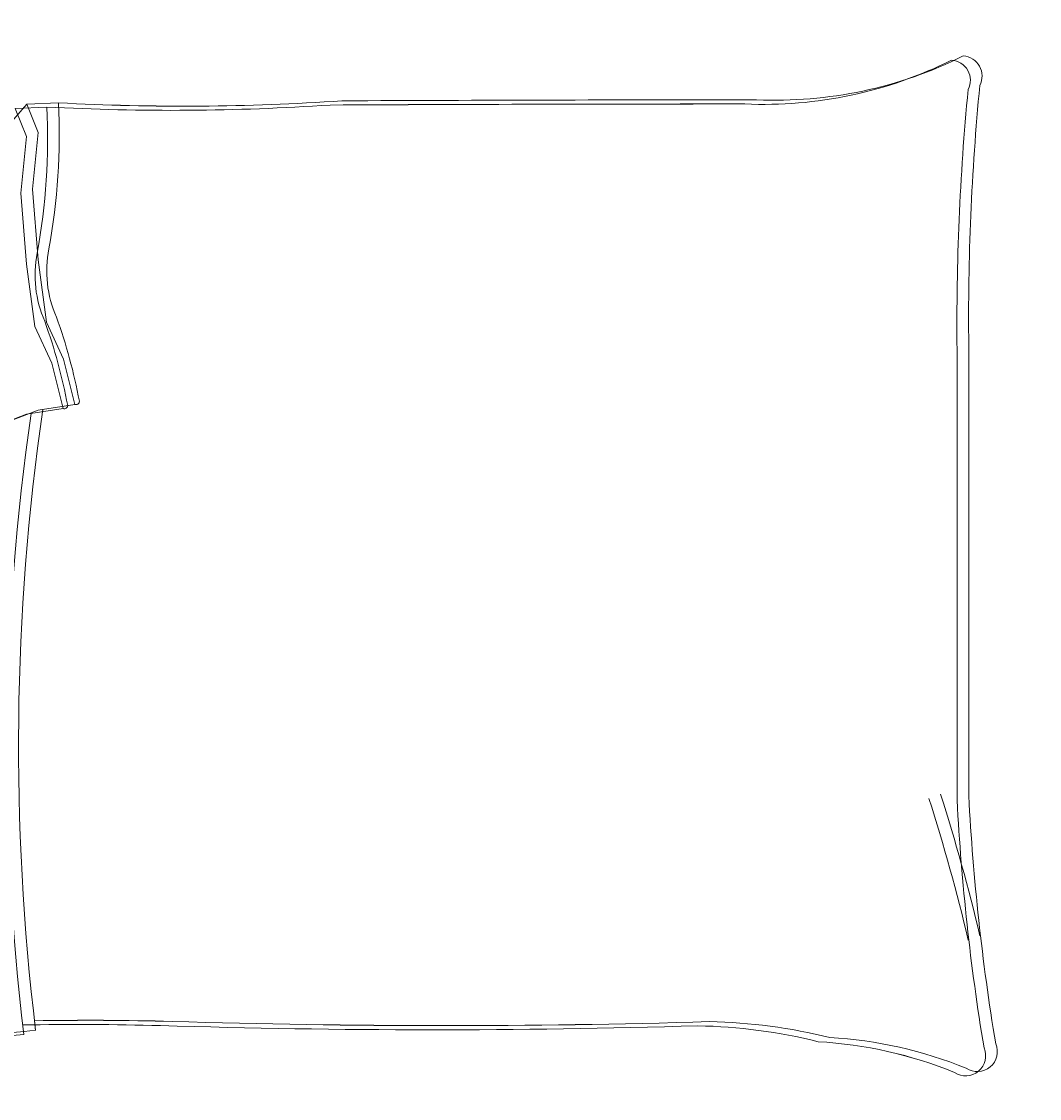
# Model space of a CAD drawing. Units: inches. Extents: x 1962 to 2771, y 1245 to 2660.
# Tile 46 of 114: x 2116 to 2160, y 2075 to 2122. Entities that reach past the tile are written whole.
import ezdxf

# ---------------------------------------------------------------- set-up
doc = ezdxf.new("R2010")
doc.units = ezdxf.units.IN
doc.layers.add('A-ANNO-DIMS', color=2, linetype='Continuous', lineweight=18)
doc.layers.add('A-FURN', color=8, linetype='Continuous', lineweight=13)
doc.styles.get("Standard").update_dxf_attribs({"font": 'arial.ttf'})
doc.dimstyles.get("Standard").update_dxf_attribs({"dimtxt": 0.18, "dimasz": 0.18, "dimexe": 0.18, "dimexo": 0.0625, "dimgap": 0.09, "dimtad": 0, "dimtih": 1, "dimtoh": 1, "dimdec": 4, "dimzin": 0, "dimdsep": 46, "dimtxsty": 'Standard', "dimcen": 0.09, "dimadec": 0, "dimazin": 0, "dimtfac": 1, "dimtdec": 4, "dimtofl": 0, "dimtmove": 0, "dimatfit": 3, "dimfxl": 1, "dimtolj": 1, "dimtzin": 0, "dimarcsym": 0})

# ---------------------------------------------------------------- blocks, each defined once
blk = doc.blocks.new('BED-PLAN')
for p, q in [((22.563, 42.207), (19.979, 39.261)), ((22.563, 42.206), (19.979, 39.261)), ((23.95, 42.27), (22.563, 42.207, 3.077)), ((23.95, 42.27), (22.563, 42.206, 3.077)), ((23.055, 40.985), (22.563, 42.207)), ((23.055, 40.985), (22.563, 42.206)), ((23.442, 42.088), (22.055, 42.025, 3.077)), ((23.442, 42.088), (22.055, 42.025, 3.077)), ((22.547, 40.803), (22.055, 42.025)), ((22.547, 40.803), (22.055, 42.025)), ((22.301, 38.341), (22.547, 40.803)), ((22.301, 38.341), (22.547, 40.803)), ((22.809, 38.523), (23.055, 40.985)), ((22.809, 38.522), (23.055, 40.985)), ((23.055, 35.445), (22.809, 38.523)), ((23.055, 35.445), (22.809, 38.522)), ((22.547, 35.263), (22.301, 38.341)), ((22.547, 35.263), (22.301, 38.341)), ((22.916, 32.555), (22.547, 35.263)), ((22.916, 32.555), (22.547, 35.263)), ((23.424, 32.737), (23.055, 35.445)), ((23.424, 32.736), (23.055, 35.445)), ((23.654, 30.955), (22.916, 32.555)), ((23.654, 30.955), (22.916, 32.555)), ((24.162, 31.136), (23.424, 32.737)), ((24.162, 31.136), (23.424, 32.736)), ((62.991, 11.975), (62.991, 31.54)), ((62.991, 11.975), (62.991, 31.54)), ((63.499, 12.157), (63.499, 31.722)), ((63.499, 12.156), (63.499, 31.722)), ((24.146, 28.985), (23.654, 30.955)), ((24.146, 28.985), (23.654, 30.955)), ((24.655, 29.167), (24.162, 31.136)), ((24.655, 29.166), (24.162, 31.136)), ((23.055, 28.92), (24.655, 29.167)), ((23.055, 28.92), (24.655, 29.166)), ((18.979, 27.385), (22.547, 28.739)), ((18.979, 27.384), (22.547, 28.739)), ((19.487, 27.566), (23.055, 28.92)), ((19.487, 27.566), (23.055, 28.92)), ((22.547, 28.739), (24.146, 28.985)), ((22.547, 28.739), (24.146, 28.985))]:
    blk.add_line(p, q)
for centre, radius, start, end in [((54.582, 60.538), 18.334, 267.4714, 296.4681), ((54.582, 60.538), 18.334, 267.4714, 296.4681), ((55.09, 60.719), 18.334, 267.4714, 296.4681), ((55.09, 60.719), 18.334, 267.4714, 296.4681), ((62.693, 43.251), 0.876, 332.6588, 86.02), ((62.693, 43.251), 0.876, 332.6588, 86.02), ((63.201, 43.433), 0.876, 332.6588, 86.02), ((63.201, 43.432), 0.876, 332.6588, 86.02), ((168.736, 32.712), 105.752, 174.4998, 180.63509), ((168.736, 32.712), 105.752, 174.4998, 180.63509), ((169.244, 32.894), 105.752, 174.4998, 180.63509), ((169.244, 32.894), 105.752, 174.4998, 180.63509), ((28.866, 144.882), 102.937, 266.97912, 273.83645), ((28.866, 144.882), 102.937, 266.97912, 273.83645), ((-4.783, 40.982), 28.761, 349.8763, 2.5657), ((-4.783, 40.982), 28.761, 349.8763, 2.5657), ((29.375, 145.064), 102.937, 266.97912, 273.83645), ((29.375, 145.063), 102.937, 266.97912, 273.83645), ((53.91, -3583.936), 3626.158, 90.002168, 90.286887), ((53.91, -3583.937), 3626.158, 90.002168, 90.286887), ((54.419, -3583.755), 3626.158, 90.002168, 90.286887), ((54.419, -3583.755), 3626.158, 90.002168, 90.286887), ((-5.291, 40.801), 28.761, 349.8763, 2.5657), ((-5.291, 40.801), 28.761, 349.8763, 2.5657), ((27.874, 34.772), 4.948, 168.6608, 203.7384), ((27.874, 34.772), 4.948, 168.6608, 203.7384), ((28.382, 34.954), 4.948, 168.6608, 203.7384), ((28.382, 34.954), 4.948, 168.6608, 203.7384), ((1.178, 24.765), 23.571, 10.6617, 19.8806), ((1.178, 24.765), 23.571, 10.6617, 19.8806), ((1.686, 24.947), 23.571, 10.6617, 19.8806), ((1.686, 24.946), 23.571, 10.6617, 19.8806), ((24.196, 29.123), 0.147, 250.2464, 1.1377), ((24.196, 29.123), 0.147, 250.2464, 1.1377), ((24.704, 29.305), 0.147, 250.2464, 1.1377), ((24.704, 29.304), 0.147, 250.2464, 1.1377), ((124.254, 14.115), 102.556, 171.78449, 186.90062), ((124.254, 14.115), 102.556, 171.78449, 186.90062), ((124.762, 14.297), 102.556, 171.78449, 186.90062), ((124.762, 14.296), 102.556, 171.78449, 186.90062), ((-18.34, -13.506), 84.623, 13.38322, 17.70533), ((-18.34, -13.507), 84.623, 13.38322, 17.70533), ((-18.848, -13.688), 84.623, 13.38322, 17.70533), ((-18.848, -13.688), 84.623, 13.38322, 17.70533), ((159.643, 17.033), 96.784, 182.99578, 189.40907), ((159.643, 17.033), 96.784, 182.99578, 189.40907), ((160.151, 17.215), 96.784, 182.99578, 189.40907), ((160.151, 17.215), 96.784, 182.99578, 189.40907), ((25.288, -132.807), 135.218, 88.4762, 91.00819), ((25.288, -132.808), 135.218, 88.4762, 91.00819), ((40.74, 385.562), 383.382, 268.22771, 271.71854), ((40.74, 385.561), 383.382, 268.22771, 271.71854), ((51.79, -21.199), 23.556, 76.0648, 88.9113), ((51.79, -21.199), 23.556, 76.0648, 88.9113), ((16.482, 67.877), 66.218, 268.72178, 275.60397), ((16.483, 67.877), 66.218, 268.72178, 275.60397), ((24.78, -132.989), 135.218, 88.4762, 91.00819), ((24.78, -132.989), 135.218, 88.4762, 91.00819), ((40.232, 385.38), 383.382, 268.22771, 271.71854), ((40.232, 385.38), 383.382, 268.22771, 271.71854), ((51.282, -21.381), 23.556, 76.0648, 88.9113), ((51.282, -21.381), 23.556, 76.0648, 88.9113), ((15.974, 67.695), 66.218, 268.72178, 275.60397), ((15.974, 67.695), 66.218, 268.72178, 275.60397), ((55.861, -17.215), 18.729, 67.9751, 86.652), ((55.861, -17.216), 18.729, 67.9751, 86.652), ((56.369, -17.034), 18.729, 67.9751, 86.652), ((56.369, -17.034), 18.729, 67.9751, 86.652), ((63.367, 0.866), 0.866, 236.1736, 23.4781), ((63.367, 0.866), 0.866, 236.1736, 23.4781), ((63.875, 1.047), 0.866, 236.1736, 23.4781), ((63.875, 1.047), 0.866, 236.1736, 23.4781)]:
    blk.add_arc(centre, radius, start, end)
blk = doc.blocks.new('*D40')
at = {"layer": 'A-ANNO-DIMS', "color": 0, "lineweight": -2, "transparency": 16777216}
for p, q in [((2072.02, 2033.906), (2072.02, 2583.474)), ((2072.2, 2583.294), (2366.02, 2583.294)), ((2660.627, 2583.294), (2366.808, 2583.294)), ((2660.807, 2524.406), (2660.807, 2583.474))]:
    blk.add_line(p, q, dxfattribs=at)
at = {"layer": 'A-ANNO-DIMS', "color": 0, "transparency": 16777216}
for points in [[(2072.2, 2583.324), (2072.2, 2583.264), (2072.02, 2583.294)], [(2660.627, 2583.324), (2660.627, 2583.264), (2660.807, 2583.294)]]:
    blk.add_solid(points, dxfattribs=at)
at = {"layer": 'Defpoints', "color": 0, "transparency": 16777216}
for p in [(2660.807, 2583.294), (2660.807, 2524.344), (2072.02, 2033.844)]:
    blk.add_point(p, dxfattribs=at)
at = {"layer": 'A-ANNO-DIMS', "color": 0, "transparency": 16777216, "insert": (2366.414, 2583.294), "char_height": 0.18, "attachment_point": 5}
blk.add_mtext('\\A1;588.8', dxfattribs=at)

msp = doc.modelspace()

# ---------------------------------------------------------------- block references
at = {"layer": 'A-FURN'}
msp.add_blockref('BED-PLAN', (2093.917, 2076.454), dxfattribs=at)

# ---------------------------------------------------------------- dimensions: what is measured, and where the dimension line sits
at = {"layer": 'A-ANNO-DIMS'}
dim = msp.add_linear_dim(base=(2660.8074, 2583.2937), p1=(2072.0204, 2033.8437), p2=(2660.8074, 2524.3437), dimstyle='Standard', override={"dimdec": 1, "dimlfac": 1, "dimrnd": 0, "dimzin": 0, "dimdsep": 46, "dimlunit": 2}, dxfattribs=at)
dim.commit()
dim.dimension.update_dxf_attribs({"geometry": '*D40', "text_midpoint": (2366.4139, 2583.2937)})

doc.saveas('drawing.dxf')
